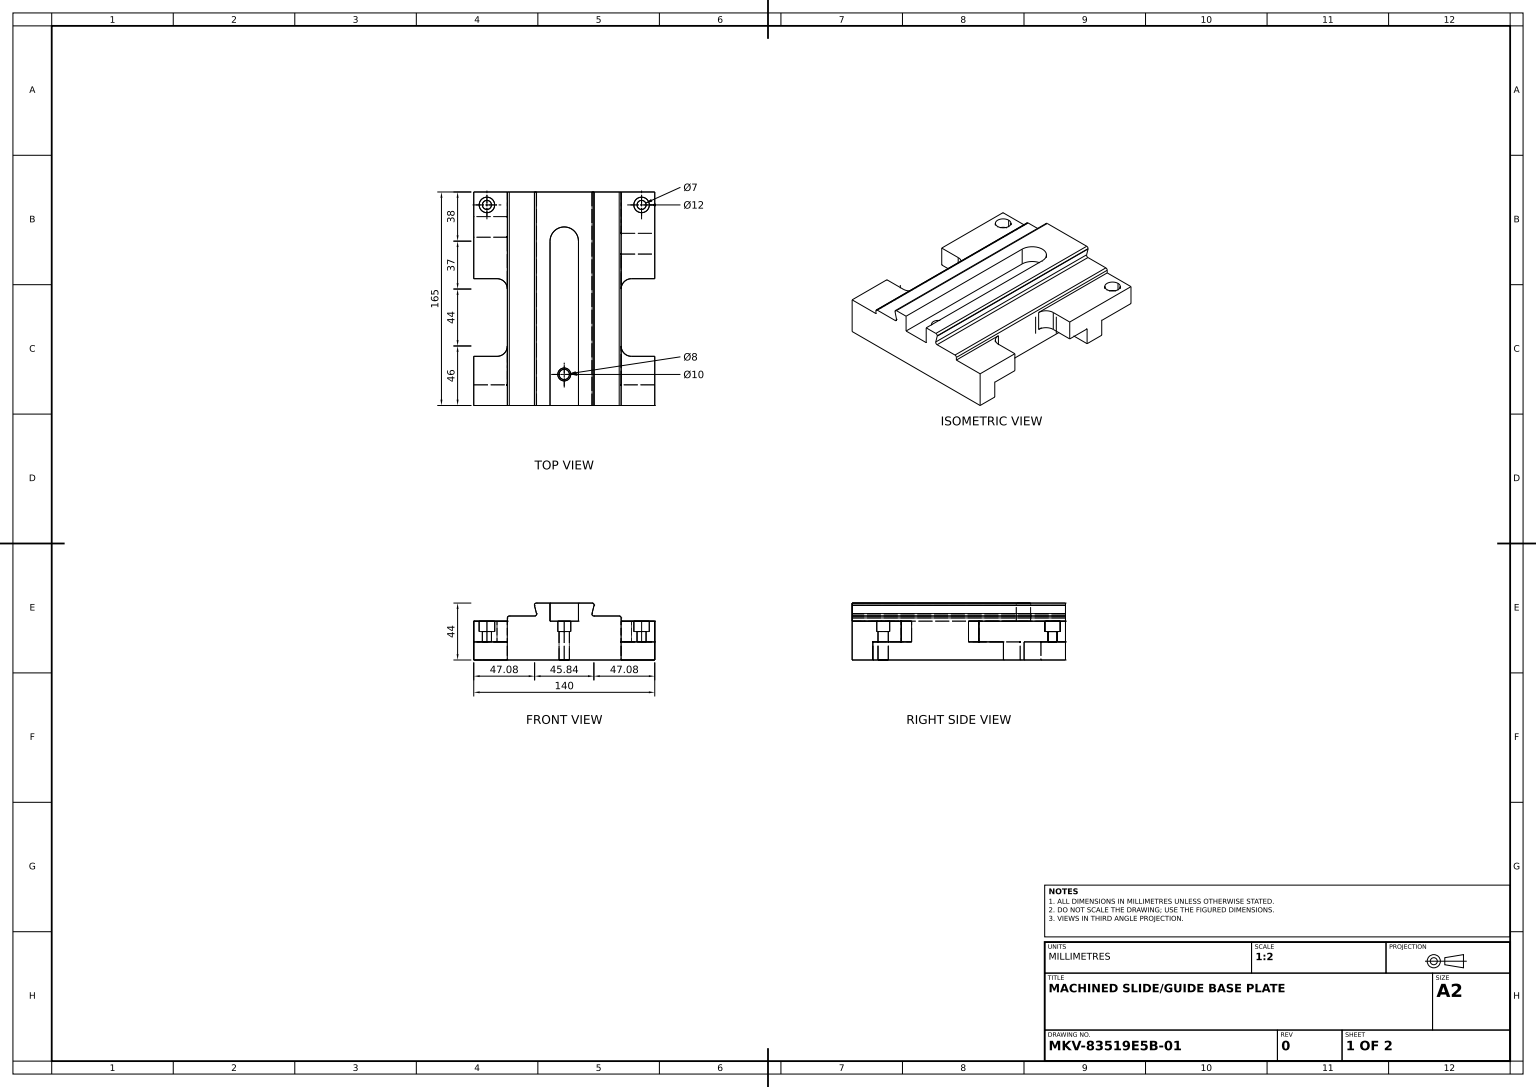
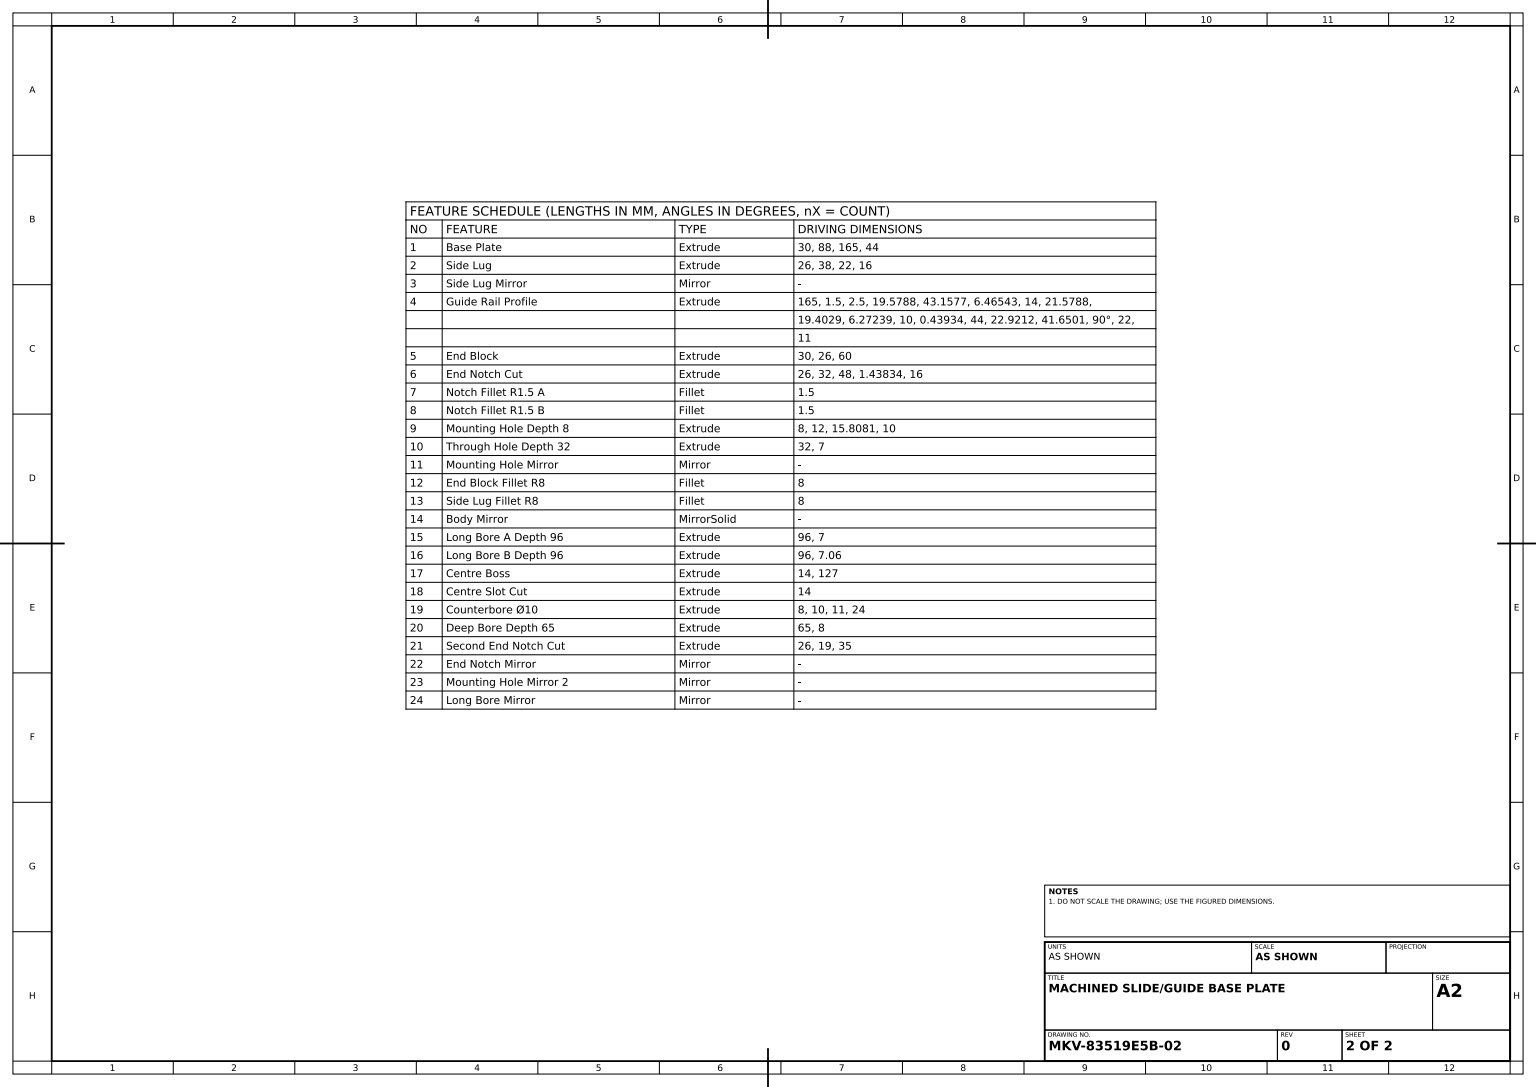
from build123d import *

# Parameters (mm, degrees)
BASE_PLATE_DEPTH            = 30
SIDE_LUG_DEPTH              = 26
GUIDE_RAIL_PROFILE_DEPTH    = 165
END_BLOCK_SKETCH_W          = 26
END_BLOCK_SKETCH_H          = 67
END_BLOCK_DEPTH             = 30
END_NOTCH_SKETCH_W          = 19
END_NOTCH_SKETCH_H          = 14
END_NOTCH_SKETCH_W_2        = 32
END_NOTCH_CUT_DEPTH         = 26
NOTCH_FILLET_R1_5_A_R       = 1.5
NOTCH_FILLET_R1_5_B_R       = 1.5
MOUNTING_HOLE_SKETCH_R      = 6
MOUNTING_HOLE_DEPTH_8_DEPTH = 8
THROUGH_HOLE_SKETCH_R       = 3.5
THROUGH_HOLE_DEPTH_32_DEPTH = 32
END_BLOCK_FILLET_R8_R       = 8
SIDE_LUG_FILLET_R8_R        = 8
LONG_BORE_A_SKETCH_R        = 3.5
LONG_BORE_A_DEPTH_96_DEPTH  = 96
LONG_BORE_B_SKETCH_R        = 3.53
LONG_BORE_B_DEPTH_96_DEPTH  = 96
CENTRE_BOSS_SKETCH_W        = 22
CENTRE_BOSS_SKETCH_H        = 38
CENTRE_BOSS_DEPTH           = 14
CENTRE_SLOT_CUT_DEPTH       = 14
COUNTERBORE_10_SKETCH_R     = 5
COUNTERBORE_10_DEPTH        = 8
DEEP_BORE_SKETCH_R          = 4
DEEP_BORE_DEPTH_65_DEPTH    = 65
SECOND_END_NOTCH_SKETCH_W   = 32
SECOND_END_NOTCH_SKETCH_H   = 14
SECOND_END_NOTCH_SKETCH_W_2 = 19
SECOND_END_NOTCH_CUT_DEPTH  = 26


with BuildPart() as part:
    # Base Plate Sketch → Base Plate (new body)
    with BuildSketch(Plane(origin=(0, 0, 0), x_dir=(1, 0, 0), z_dir=(0, 1, 0))):
        Polygon((44, 0), (44, -82.5), (-44, -82.5), (-44, 82.5), (44, 82.5), align=None)
    extrude(amount=-BASE_PLATE_DEPTH)

    # Side Lug Sketch → Side Lug (add)
    with BuildSketch(Plane(origin=(44, 0, 0), x_dir=(0, 0, -1), z_dir=(1, 0, 0))):
        Polygon((-82.5, -30), (-82.5, 0), (-44.5, 0), (-44.5, -16), (-66.5, -16), (-66.5, -30), align=None)
    side_lug = extrude(amount=SIDE_LUG_DEPTH)

    # Side Lug Mirror: Side Lug across plane
    add(side_lug.mirror(Plane(origin=(0, 0, 0), x_dir=(0, 0, 1), z_dir=(1, 0, 0))))


with BuildPart() as guide_rail_profile_tool:
    # Guide Rail Profile Sketch → Guide Rail Profile (new body)
    with BuildSketch(Plane.XY.offset(82.5)):
        with BuildLine():
            Line((11, 14), (11, 0))
            Line((11, 0), (44, 0))
            Line((44, 0), (44, 2.5))
            ThreePointArc((44, 2.5), (43.560660172, 3.560660172), (42.5, 4))
            Line((42.5, 4), (22.92116461, 4))
            ThreePointArc((22.92116461, 4), (21.738856453, 4.576881686), (21.465950859, 5.863803438))
            Line((21.465950859, 5.863803438), (23.034049141, 12.136196562))
            ThreePointArc((23.034049141, 12.136196562), (22.761143547, 13.423118314), (21.57883539, 14))
            Line((21.57883539, 14), (11, 14))
        make_face()
        with BuildLine():
            Line((-44, 7.32e-07), (-11, 0))
            Line((-11, 0), (-11, 14))
            Line((-11, 14), (-21.57883539, 14))
            ThreePointArc((-21.57883539, 14), (-22.761143547, 13.423118314), (-23.034049141, 12.136196562))
            Line((-23.034049141, 12.136196562), (-21.465950859, 5.863803438))
            ThreePointArc((-21.465950859, 5.863803438), (-21.738856678, 4.576881398), (-22.921165341, 4))
            Line((-22.921165341, 4), (-42.500000732, 4))
            ThreePointArc((-42.500000732, 4), (-43.560660172, 3.560660172), (-44, 2.500000732))
            Line((-44, 2.500000732), (-44, 7.32e-07))
        make_face()
    extrude(amount=-GUIDE_RAIL_PROFILE_DEPTH)


with BuildPart() as part_1:
    add(part.part)


with BuildPart() as part_2:
    # Guide Rail Profile: joined with guide_rail_profile_tool
    add(part_1.part.fuse(guide_rail_profile_tool.part, tol=0.00001))

    # End Block Sketch → End Block (add)
    with BuildSketch(Plane(origin=(0, 0, 0), x_dir=(1, 0, 0), z_dir=(0, 1, 0))):
        with Locations((-57, 49)):
            Rectangle(END_BLOCK_SKETCH_W, END_BLOCK_SKETCH_H)
    end_block = extrude(amount=-END_BLOCK_DEPTH)

    # End Notch Sketch → End Notch Cut (cut)
    with BuildSketch(Plane.ZY.offset(70)):
        with Locations((-25, -23)):
            Rectangle(END_NOTCH_SKETCH_W, END_NOTCH_SKETCH_H)
        with Locations((-66.5, -23)):
            Rectangle(END_NOTCH_SKETCH_W_2, END_NOTCH_SKETCH_H)
    end_notch_cut = extrude(amount=-END_NOTCH_CUT_DEPTH, mode=Mode.SUBTRACT)

    # Notch Fillet R1.5 A
    notch_fillet_r1_5_a_edges = [part_2.edges().sort_by_distance(p)[0] for p in [
        (-57, -16, -50.5),
    ]]
    fillet(notch_fillet_r1_5_a_edges, radius=NOTCH_FILLET_R1_5_A_R)

    # Notch Fillet R1.5 B
    notch_fillet_r1_5_b_edges = [part_2.edges().sort_by_distance(p)[0] for p in [
        (-57, -16, -34.5),
    ]]
    fillet(notch_fillet_r1_5_b_edges, radius=NOTCH_FILLET_R1_5_B_R)

    # Mounting Hole Sketch → Mounting Hole Depth 8 (cut)
    with BuildSketch(Plane(origin=(0, 0, 0), x_dir=(1, 0, 0), z_dir=(0, 1, 0))):
        with Locations(Location((-59.808082778, 72.5, 0), (0, 0, 270))):
            Circle(MOUNTING_HOLE_SKETCH_R)
    mounting_hole_depth_8 = extrude(amount=-MOUNTING_HOLE_DEPTH_8_DEPTH, mode=Mode.SUBTRACT)

    # Through Hole Sketch → Through Hole Depth 32 (cut)
    with BuildSketch(Plane(origin=(0, 0, 0), x_dir=(1, 0, 0), z_dir=(0, 1, 0))):
        with Locations(Location((-59.808082778, 72.5, 0), (0, 0, 270))):
            Circle(THROUGH_HOLE_SKETCH_R)
    extrude(amount=-THROUGH_HOLE_DEPTH_32_DEPTH, mode=Mode.SUBTRACT)

    # Mounting Hole Mirror: End Block, Mounting Hole Depth 8 across plane
    add(end_block.mirror(Plane(origin=(0, 0, 0), x_dir=(0, 0, 1), z_dir=(1, 0, 0))))
    add(mounting_hole_depth_8.mirror(Plane(origin=(0, 0, 0), x_dir=(0, 0, 1), z_dir=(1, 0, 0))), mode=Mode.SUBTRACT)

    # End Block Fillet R8
    end_block_fillet_r8_edges = [part_2.edges().sort_by_distance(p)[0] for p in [
        (-44, -8, -15.5),
    ]]
    fillet(end_block_fillet_r8_edges, radius=END_BLOCK_FILLET_R8_R)

    # Side Lug Fillet R8
    side_lug_fillet_r8_edges = [part_2.edges().sort_by_distance(p)[0] for p in [
        (-44, -8, 44.5),
    ]]
    fillet(side_lug_fillet_r8_edges, radius=SIDE_LUG_FILLET_R8_R)

    # Body Mirror: part across plane


with BuildPart() as part_3:
    add(part_2.part)
    add(part_2.part.mirror(Plane(origin=(0, 0, 0), x_dir=(0, 0, 1), z_dir=(1, 0, 0))))

    # Long Bore A Sketch → Long Bore A Depth 96 (cut)
    with BuildSketch(Plane(origin=(0, -8, 0), x_dir=(1, 0, 0), z_dir=(0, 1, 0))):
        with Locations(Location((-59.808082778, 72.5, 0), (0, 0, 270))):
            Circle(LONG_BORE_A_SKETCH_R)
    long_bore_a_depth_96 = extrude(amount=-LONG_BORE_A_DEPTH_96_DEPTH, mode=Mode.SUBTRACT)

    # Long Bore B Sketch → Long Bore B Depth 96 (cut)
    with BuildSketch(Plane.XZ.offset(30)):
        with Locations(Location((59.808082778, -72.5, 0), (0, 0, 270))):
            Circle(LONG_BORE_B_SKETCH_R)
    extrude(amount=-LONG_BORE_B_DEPTH_96_DEPTH, mode=Mode.SUBTRACT)

    # Centre Boss Sketch → Centre Boss (add)
    with BuildSketch(Plane(origin=(0, 14, 0), x_dir=(1, 0, 0), z_dir=(0, 1, 0))):
        with Locations((0, 63.5)):
            Rectangle(CENTRE_BOSS_SKETCH_W, CENTRE_BOSS_SKETCH_H)
    extrude(amount=-CENTRE_BOSS_DEPTH)

    # Centre Slot Sketch → Centre Slot Cut (cut)
    with BuildSketch(Plane(origin=(0, 14, 0), x_dir=(1, 0, 0), z_dir=(0, 1, 0))):
        with BuildLine():
            Line((-11, 44.5), (11, 44.5))
            ThreePointArc((11, 44.5), (0, 55.5), (-11, 44.5))
        make_face()
    extrude(amount=-CENTRE_SLOT_CUT_DEPTH, mode=Mode.SUBTRACT)

    # Counterbore Ø10 Sketch → Counterbore Ø10 (cut)
    with BuildSketch(Plane(origin=(0, 0, 0), x_dir=(1, 0, 0), z_dir=(0, 1, 0))):
        with Locations(Location((0, -58.5, 0), (0, 0, 270))):
            Circle(COUNTERBORE_10_SKETCH_R)
    extrude(amount=-COUNTERBORE_10_DEPTH, mode=Mode.SUBTRACT)

    # Deep Bore Sketch → Deep Bore Depth 65 (cut)
    with BuildSketch(Plane(origin=(0, -8, 0), x_dir=(1, 0, 0), z_dir=(0, 1, 0))):
        with Locations(Location((0, -58.5, 0), (0, 0, 270))):
            Circle(DEEP_BORE_SKETCH_R)
    extrude(amount=-DEEP_BORE_DEPTH_65_DEPTH, mode=Mode.SUBTRACT)

    # Second End Notch Sketch → Second End Notch Cut (cut)
    with BuildSketch(Plane.ZY.offset(70)):
        with Locations((-31.5, -23)):
            Rectangle(SECOND_END_NOTCH_SKETCH_W, SECOND_END_NOTCH_SKETCH_H)
        with Locations((-73, -23)):
            Rectangle(SECOND_END_NOTCH_SKETCH_W_2, SECOND_END_NOTCH_SKETCH_H)
    extrude(amount=-SECOND_END_NOTCH_CUT_DEPTH, mode=Mode.SUBTRACT)

    # End Notch Mirror: End Block, End Notch Cut across plane
    add(end_block.mirror(Plane(origin=(0, 0, 0), x_dir=(0, 0, 1), z_dir=(1, 0, 0))))
    add(end_notch_cut.mirror(Plane(origin=(0, 0, 0), x_dir=(0, 0, 1), z_dir=(1, 0, 0))), mode=Mode.SUBTRACT)

    # Mounting Hole Mirror 2: Mounting Hole Depth 8 across plane
    add(mounting_hole_depth_8.mirror(Plane(origin=(0, 0, 0), x_dir=(0, 0, 1), z_dir=(1, 0, 0))), mode=Mode.SUBTRACT)

    # Long Bore Mirror: Long Bore A Depth 96 across plane
    add(long_bore_a_depth_96.mirror(Plane(origin=(0, 0, 0), x_dir=(0, 0, 1), z_dir=(1, 0, 0))), mode=Mode.SUBTRACT)


solid = part_3.part
